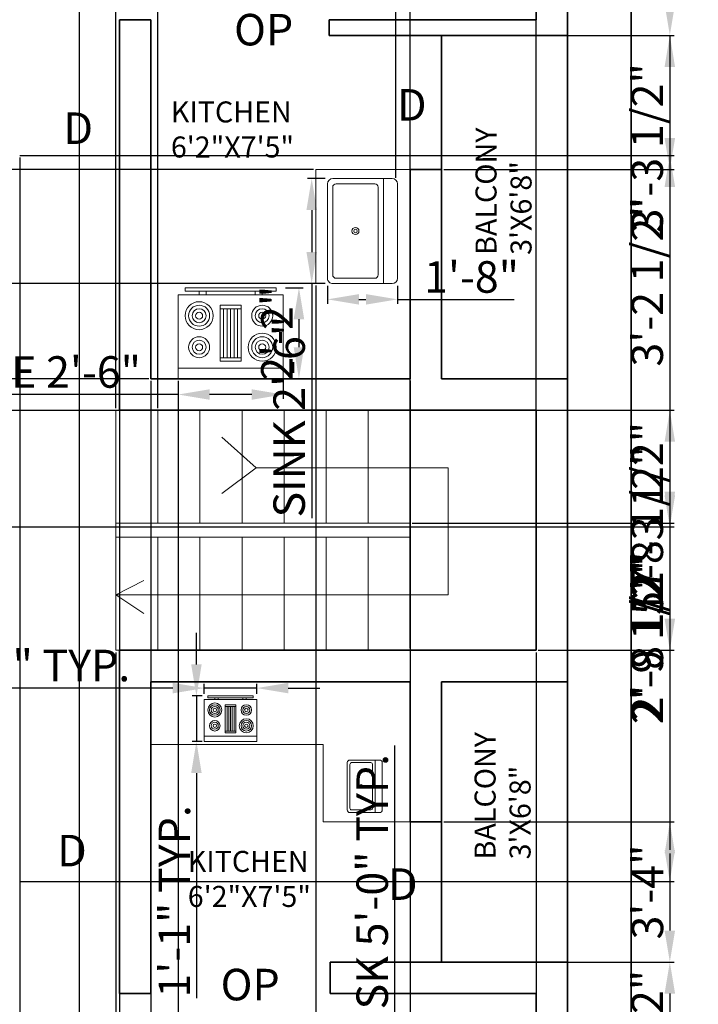
# Model space of a CAD drawing. Units: inches. Extents: x 53076 to 53578, y 41072 to 41816.
# Tile 3 of 4: x 53326 to 53520, y 41279 to 41560. Entities that reach past the tile are written whole.
import ezdxf

# ---------------------------------------------------------------- set-up
doc = ezdxf.new("R2010")
doc.units = ezdxf.units.IN
for name, color, linetype, lineweight in [('A-ANNO-DIMS', 2, 'Continuous', 18), ('A-ANNO-TEXT', 7, 'Continuous', 18), ('A-ANNO-TTLB', 7, 'Continuous', 35), ('A-AREA-IDEN', 7, 'Continuous', 18), ('A-DOOR', 3, 'Continuous', 25), ('A-EQPM', 8, 'Continuous', 18), ('A-FLOR-CASE', 9, 'Continuous', 18), ('A-FLOR-FIXT', 9, 'Continuous', 18), ('A-FLOR-STRS', 7, 'Continuous', 18), ('A-WALL', 7, 'Continuous', 35)]:
    doc.layers.add(name, color=color, linetype=linetype, lineweight=lineweight)
doc.styles.get("Standard").update_dxf_attribs({"font": 'arial.ttf'})
doc.dimstyles.new('ISO-25', dxfattribs={"dimtxt": 9, "dimasz": 9, "dimexe": 1.25, "dimexo": 0.625, "dimtad": 1, "dimdec": 1, "dimrnd": 9, "dimlunit": 3, "dimtxsty": 'Standard', "dimcen": 2.5, "dimadec": 0, "dimazin": 0, "dimtfac": 1, "dimtdec": 1, "dimtmove": 0, "dimatfit": 3, "dimfxl": 1, "dimarcsym": 0})

# ---------------------------------------------------------------- blocks, each defined once
blk = doc.blocks.new('Sink-single - 30 in top')
blk.add_line((-15, -3.999996), (15, -3.999996))
for points in [[(-13.5, 0), (13.5, 0)], [(-15, -18.499996), (-15, -1.5)], [(15, -1.5), (15, -18.499996)], [(-12.5, -5.499996), (12.5, -5.499996)], [(-13.5, -17.499996), (-13.5, -6.499996)], [(13.5, -6.499996), (13.5, -17.499996)], [(12.5, -18.499996), (-12.5, -18.499996)], [(13.5, -19.999996), (-13.5, -19.999996)]]:
    blk.add_lwpolyline(points)
for radius in [1, 0.5]:
    blk.add_circle((0, -11.999996), radius)
for centre, radius, start, end in [((-13.5, -1.5), 1.5, 90, 180), ((13.5, -1.5), 1.5, 0, 90), ((-12.5, -6.499996), 1, 90, 180), ((12.5, -6.499996), 1, 0, 90), ((-13.5, -18.499996), 1.5, 180, 270), ((-12.5, -17.499996), 1, 180, 270), ((12.5, -17.499996), 1, 270, 0), ((13.5, -18.499996), 1.5, 270, 0)]:
    blk.add_arc(centre, radius, start, end)
blk = doc.blocks.new('Range-Oven - 30 in top')
for p, q in [((0, -3), (30, -3)), ((12, -6), (18, -6)), ((13, -20), (13, -6)), ((14, -6), (14, -20)), ((15, -20), (15, -6)), ((16, -6), (16, -20)), ((17, -20), (17, -6)), ((18, -20), (12, -20)), ((6, -24), (6, -25)), ((8, -25), (8, -24)), ((22, -25), (22, -24)), ((24, -24), (24, -25))]:
    blk.add_line(p, q)
for points in [[(0, -24), (0, 0), (30, 0), (30, -24)], [(12, -21), (12, -5), (18, -5), (18, -21)], [(2, -26), (2, -25), (28, -25), (28, -26)]]:
    blk.add_lwpolyline(points, close=True)
for centre, radius in [((6, -9), 4), ((6, -9), 3), ((6, -9), 2), ((6, -9), 1), ((24, -9), 3), ((24, -9), 2), ((24, -9), 1), ((24, -18), 4), ((6, -18), 3), ((6, -18), 2), ((24, -18), 3), ((24, -18), 2), ((6, -18), 1), ((24, -18), 1)]:
    blk.add_circle(centre, radius)
blk = doc.blocks.new('DOOR-ENTRY-28_5IN')
blk.add_line((0, 0), (28.5, 0))
blk = doc.blocks.new('*D16')
at = {"layer": 'A-ANNO-DIMS', "color": 0, "lineweight": -2, "transparency": 16777216}
for p, q in [((53413.6, 41514.33), (53408.47, 41514.33)), ((53409.72, 41505.33), (53409.72, 41493.33)), ((53413.6, 41484.33), (53408.47, 41484.33)), ((53409.72, 41484.33), (53409.72, 41417.36))]:
    blk.add_line(p, q, dxfattribs=at)
at = {"layer": 'A-ANNO-DIMS', "color": 0, "transparency": 16777216}
for points in [[(53408.22, 41505.33), (53411.22, 41505.33), (53409.72, 41514.33)], [(53408.22, 41493.33), (53411.22, 41493.33), (53409.72, 41484.33)]]:
    blk.add_solid(points, dxfattribs=at)
at = {"layer": 'Defpoints', "color": 0, "transparency": 16777216}
for p in [(53414.22, 41514.33), (53409.72, 41484.33), (53414.22, 41484.33)]:
    blk.add_point(p, dxfattribs=at)
at = {"layer": 'A-ANNO-DIMS', "color": 0, "transparency": 16777216, "insert": (53404.44, 41446.35), "char_height": 9, "attachment_point": 5, "rotation": 90}
blk.add_mtext('SINK 2\'-6"', dxfattribs=at)
blk = doc.blocks.new('*D17')
at = {"layer": 'A-ANNO-DIMS', "color": 0, "lineweight": -2, "transparency": 16777216}
for p, q in [((53414.22, 41483.71), (53414.22, 41478.58)), ((53434.22, 41483.71), (53434.22, 41478.58)), ((53423.22, 41479.83), (53425.22, 41479.83)), ((53434.22, 41479.83), (53467.55, 41479.83))]:
    blk.add_line(p, q, dxfattribs=at)
at = {"layer": 'A-ANNO-DIMS', "color": 0, "transparency": 16777216}
for points in [[(53423.22, 41481.33), (53423.22, 41478.33), (53414.22, 41479.83)], [(53425.22, 41481.33), (53425.22, 41478.33), (53434.22, 41479.83)]]:
    blk.add_solid(points, dxfattribs=at)
at = {"layer": 'Defpoints', "color": 0, "transparency": 16777216}
for p in [(53414.22, 41484.33), (53434.22, 41484.33), (53434.22, 41479.83)]:
    blk.add_point(p, dxfattribs=at)
at = {"layer": 'A-ANNO-DIMS', "color": 0, "transparency": 16777216, "insert": (53455.38, 41485.05), "char_height": 9, "attachment_point": 5}
blk.add_mtext('1\'-8"', dxfattribs=at)
blk = doc.blocks.new('*D20')
at = {"layer": 'A-ANNO-DIMS', "color": 0, "lineweight": -2, "transparency": 16777216}
for p, q in [((53371.57, 41456.53), (53371.57, 41451.41)), ((53401.57, 41456.53), (53401.57, 41451.41)), ((53371.57, 41452.66), (53289.65, 41452.66)), ((53392.57, 41452.66), (53380.57, 41452.66))]:
    blk.add_line(p, q, dxfattribs=at)
at = {"layer": 'A-ANNO-DIMS', "color": 0, "transparency": 16777216}
for points in [[(53380.57, 41454.16), (53380.57, 41451.16), (53371.57, 41452.66)], [(53392.57, 41454.16), (53392.57, 41451.16), (53401.57, 41452.66)]]:
    blk.add_solid(points, dxfattribs=at)
at = {"layer": 'Defpoints', "color": 0, "transparency": 16777216}
for p in [(53371.57, 41457.16), (53401.57, 41457.16), (53371.57, 41452.66)]:
    blk.add_point(p, dxfattribs=at)
at = {"layer": 'A-ANNO-DIMS', "color": 0, "transparency": 16777216, "insert": (53326.11, 41457.93), "char_height": 9, "attachment_point": 5}
blk.add_mtext('RANGE 2\'-6"', dxfattribs=at)
blk = doc.blocks.new('*D21')
at = {"layer": 'A-ANNO-DIMS', "color": 0, "lineweight": -2, "transparency": 16777216}
for p, q in [((53402.19, 41483.16), (53407.32, 41483.16)), ((53406.07, 41474.16), (53406.07, 41466.16)), ((53402.19, 41457.16), (53407.32, 41457.16))]:
    blk.add_line(p, q, dxfattribs=at)
at = {"layer": 'A-ANNO-DIMS', "color": 0, "transparency": 16777216}
for points in [[(53404.57, 41474.16), (53407.57, 41474.16), (53406.07, 41483.16)], [(53404.57, 41466.16), (53407.57, 41466.16), (53406.07, 41457.16)]]:
    blk.add_solid(points, dxfattribs=at)
at = {"layer": 'Defpoints', "color": 0, "transparency": 16777216}
for p in [(53401.57, 41483.16), (53401.57, 41457.16), (53406.07, 41457.16)]:
    blk.add_point(p, dxfattribs=at)
at = {"layer": 'A-ANNO-DIMS', "color": 0, "transparency": 16777216, "insert": (53400.92, 41470.16), "char_height": 9, "attachment_point": 5, "rotation": 90}
blk.add_mtext('2\'-2"', dxfattribs=at)
blk = doc.blocks.new('*D22')
at = {"layer": 'A-ANNO-DIMS', "color": 0, "lineweight": -2, "transparency": 16777216}
for p, q in [((53379.04, 41367.23), (53379.04, 41370.11)), ((53394.04, 41367.23), (53394.04, 41370.11)), ((53370.04, 41368.86), (53257.19, 41368.86)), ((53394.04, 41368.86), (53379.04, 41368.86)), ((53403.04, 41368.86), (53412.04, 41368.86))]:
    blk.add_line(p, q, dxfattribs=at)
at = {"layer": 'A-ANNO-DIMS', "color": 0, "transparency": 16777216}
for points in [[(53370.04, 41370.36), (53370.04, 41367.36), (53379.04, 41368.86)], [(53403.04, 41370.36), (53403.04, 41367.36), (53394.04, 41368.86)]]:
    blk.add_solid(points, dxfattribs=at)
at = {"layer": 'Defpoints', "color": 0, "transparency": 16777216}
for p in [(53379.04, 41368.86), (53379.04, 41366.61), (53394.04, 41366.61)]:
    blk.add_point(p, dxfattribs=at)
at = {"layer": 'A-ANNO-DIMS', "color": 0, "transparency": 16777216, "insert": (53309.12, 41374.14), "char_height": 9, "attachment_point": 5}
blk.add_mtext('RANGE 1\'-3" TYP.', dxfattribs=at)
blk = doc.blocks.new('*D23')
at = {"layer": 'A-ANNO-DIMS', "color": 0, "lineweight": -2, "transparency": 16777216}
for p, q in [((53376.79, 41375.61), (53376.79, 41384.61)), ((53378.42, 41366.61), (53375.54, 41366.61)), ((53376.79, 41366.61), (53376.79, 41353.61)), ((53378.42, 41353.61), (53375.54, 41353.61)), ((53376.79, 41344.61), (53376.79, 41280.35))]:
    blk.add_line(p, q, dxfattribs=at)
at = {"layer": 'A-ANNO-DIMS', "color": 0, "transparency": 16777216}
for points in [[(53375.29, 41375.61), (53378.29, 41375.61), (53376.79, 41366.61)], [(53375.29, 41344.61), (53378.29, 41344.61), (53376.79, 41353.61)]]:
    blk.add_solid(points, dxfattribs=at)
at = {"layer": 'Defpoints', "color": 0, "transparency": 16777216}
for p in [(53379.04, 41366.61), (53376.79, 41353.61), (53379.04, 41353.61)]:
    blk.add_point(p, dxfattribs=at)
at = {"layer": 'A-ANNO-DIMS', "color": 0, "transparency": 16777216, "insert": (53371.65, 41307.98), "char_height": 9, "attachment_point": 5, "rotation": 90}
blk.add_mtext('1\'-1" TYP.', dxfattribs=at)
blk = doc.blocks.new('*D28')
at = {"layer": 'A-ANNO-DIMS', "color": 0, "lineweight": -2, "transparency": 16777216}
for p, q in [((53433.43, 41250.06), (53433.43, 41352.45)), ((53425.06, 41250.06), (53434.68, 41250.06)), ((53433.43, 41199.06), (53433.43, 41241.06)), ((53425.06, 41190.06), (53434.68, 41190.06))]:
    blk.add_line(p, q, dxfattribs=at)
at = {"layer": 'A-ANNO-DIMS', "color": 0, "transparency": 16777216}
for points in [[(53431.93, 41241.06), (53434.93, 41241.06), (53433.43, 41250.06)], [(53431.93, 41199.06), (53434.93, 41199.06), (53433.43, 41190.06)]]:
    blk.add_solid(points, dxfattribs=at)
at = {"layer": 'Defpoints', "color": 0, "transparency": 16777216}
for p in [(53424.43, 41250.06), (53433.43, 41250.06), (53424.43, 41190.06)]:
    blk.add_point(p, dxfattribs=at)
at = {"layer": 'A-ANNO-DIMS', "color": 0, "transparency": 16777216, "insert": (53428.16, 41305.75), "char_height": 9, "attachment_point": 5, "rotation": 90}
blk.add_mtext('DESK 5\'-0" TYP.', dxfattribs=at)
blk = doc.blocks.new('*D32')
at = {"layer": 'A-ANNO-DIMS', "color": 0, "lineweight": -2, "transparency": 16777216}
for p, q in [((53483.43, 41594.51), (53513.26, 41594.51)), ((53512.01, 41585.51), (53512.01, 41564.16)), ((53483.43, 41555.16), (53513.26, 41555.16)), ((53512.01, 41555.16), (53512.01, 41500.02))]:
    blk.add_line(p, q, dxfattribs=at)
at = {"layer": 'A-ANNO-DIMS', "color": 0, "transparency": 16777216}
for points in [[(53510.51, 41585.51), (53513.51, 41585.51), (53512.01, 41594.51)], [(53510.51, 41564.16), (53513.51, 41564.16), (53512.01, 41555.16)]]:
    blk.add_solid(points, dxfattribs=at)
at = {"layer": 'Defpoints', "color": 0, "transparency": 16777216}
for p in [(53482.81, 41594.51), (53482.81, 41555.16), (53512.01, 41555.16)]:
    blk.add_point(p, dxfattribs=at)
at = {"layer": 'A-ANNO-DIMS', "color": 0, "transparency": 16777216, "insert": (53506.72, 41523.09), "char_height": 9, "attachment_point": 5, "rotation": 90}
blk.add_mtext('3\'-3 1/2"', dxfattribs=at)
blk = doc.blocks.new('*D33')
at = {"layer": 'A-ANNO-DIMS', "color": 0, "lineweight": -2, "transparency": 16777216}
for p, q in [((53474.43, 41448.16), (53513.26, 41448.16)), ((53512.01, 41439.16), (53512.01, 41388.66)), ((53474.43, 41379.66), (53513.26, 41379.66))]:
    blk.add_line(p, q, dxfattribs=at)
at = {"layer": 'A-ANNO-DIMS', "color": 0, "transparency": 16777216}
for points in [[(53510.51, 41439.16), (53513.51, 41439.16), (53512.01, 41448.16)], [(53510.51, 41388.66), (53513.51, 41388.66), (53512.01, 41379.66)]]:
    blk.add_solid(points, dxfattribs=at)
at = {"layer": 'Defpoints', "color": 0, "transparency": 16777216}
for p in [(53473.81, 41448.16), (53473.81, 41379.66), (53512.01, 41379.66)]:
    blk.add_point(p, dxfattribs=at)
at = {"layer": 'A-ANNO-DIMS', "color": 0, "transparency": 16777216, "insert": (53506.73, 41413.91), "char_height": 9, "attachment_point": 5, "rotation": 90}
blk.add_mtext('5\'-8 1/2"', dxfattribs=at)
blk = doc.blocks.new('*D34')
at = {"layer": 'A-ANNO-DIMS', "color": 0, "lineweight": -2, "transparency": 16777216}
for p, q in [((53353.81, 41379.03), (53353.81, 41122.21)), ((53473.81, 41379.03), (53473.81, 41122.21)), ((53362.81, 41123.46), (53464.81, 41123.46))]:
    blk.add_line(p, q, dxfattribs=at)
at = {"layer": 'A-ANNO-DIMS', "color": 0, "transparency": 16777216}
for points in [[(53362.81, 41124.96), (53362.81, 41121.96), (53353.81, 41123.46)], [(53464.81, 41124.96), (53464.81, 41121.96), (53473.81, 41123.46)]]:
    blk.add_solid(points, dxfattribs=at)
at = {"layer": 'Defpoints', "color": 0, "transparency": 16777216}
for p in [(53353.81, 41379.66), (53473.81, 41379.66), (53473.81, 41123.46)]:
    blk.add_point(p, dxfattribs=at)
at = {"layer": 'A-ANNO-DIMS', "color": 0, "transparency": 16777216, "insert": (53413.81, 41128.68), "char_height": 9, "attachment_point": 5}
blk.add_mtext('10\'-0"', dxfattribs=at)
blk = doc.blocks.new('*D35')
at = {"layer": 'A-ANNO-DIMS', "color": 0, "lineweight": -2, "transparency": 16777216}
for p, q in [((53483.43, 41290.66), (53513.26, 41290.66)), ((53512.01, 41281.66), (53512.01, 41246.92)), ((53483.43, 41237.92), (53513.26, 41237.92))]:
    blk.add_line(p, q, dxfattribs=at)
at = {"layer": 'A-ANNO-DIMS', "color": 0, "transparency": 16777216}
for points in [[(53510.51, 41281.66), (53513.51, 41281.66), (53512.01, 41290.66)], [(53510.51, 41246.92), (53513.51, 41246.92), (53512.01, 41237.92)]]:
    blk.add_solid(points, dxfattribs=at)
at = {"layer": 'Defpoints', "color": 0, "transparency": 16777216}
for p in [(53482.81, 41290.66), (53482.81, 41237.92), (53512.01, 41237.92)]:
    blk.add_point(p, dxfattribs=at)
at = {"layer": 'A-ANNO-DIMS', "color": 0, "transparency": 16777216, "insert": (53506.73, 41264.29), "char_height": 9, "attachment_point": 5, "rotation": 90}
blk.add_mtext('4\'-4 1/2"', dxfattribs=at)
blk = doc.blocks.new('*D37')
at = {"layer": 'A-ANNO-DIMS', "color": 0, "lineweight": -2, "transparency": 16777216}
for p, q in [((53326.31, 41520.3), (53326.31, 41122.21)), ((53354.81, 41520.3), (53354.81, 41122.21)), ((53335.31, 41123.46), (53345.81, 41123.46)), ((53354.81, 41123.46), (53410.11, 41123.46))]:
    blk.add_line(p, q, dxfattribs=at)
at = {"layer": 'A-ANNO-DIMS', "color": 0, "transparency": 16777216}
for points in [[(53335.31, 41124.96), (53335.31, 41121.96), (53326.31, 41123.46)], [(53345.81, 41124.96), (53345.81, 41121.96), (53354.81, 41123.46)]]:
    blk.add_solid(points, dxfattribs=at)
at = {"layer": 'Defpoints', "color": 0, "transparency": 16777216}
for p in [(53326.31, 41520.92), (53354.81, 41520.92), (53354.81, 41123.46)]:
    blk.add_point(p, dxfattribs=at)
at = {"layer": 'A-ANNO-DIMS', "color": 0, "transparency": 16777216, "insert": (53386.96, 41128.73), "char_height": 9, "attachment_point": 5}
blk.add_mtext('2\'-4 1/2"', dxfattribs=at)
blk = doc.blocks.new('*D38')
at = {"layer": 'A-ANNO-DIMS', "color": 0, "lineweight": -2, "transparency": 16777216}
for p, q in [((53326.93, 41520.92), (53513.26, 41520.92)), ((53512.01, 41511.92), (53512.01, 41322.66)), ((53326.93, 41313.66), (53513.26, 41313.66))]:
    blk.add_line(p, q, dxfattribs=at)
at = {"layer": 'A-ANNO-DIMS', "color": 0, "transparency": 16777216}
for points in [[(53510.51, 41511.92), (53513.51, 41511.92), (53512.01, 41520.92)], [(53510.51, 41322.66), (53513.51, 41322.66), (53512.01, 41313.66)]]:
    blk.add_solid(points, dxfattribs=at)
at = {"layer": 'Defpoints', "color": 0, "transparency": 16777216}
for p in [(53326.31, 41520.92), (53326.31, 41313.66), (53512.01, 41313.66)]:
    blk.add_point(p, dxfattribs=at)
at = {"layer": 'A-ANNO-DIMS', "color": 0, "transparency": 16777216, "insert": (53506.72, 41417.29), "char_height": 9, "attachment_point": 5, "rotation": 90}
blk.add_mtext('17\'-3 1/2"', dxfattribs=at)
blk = doc.blocks.new('*D53')
at = {"layer": 'A-ANNO-DIMS', "color": 0, "lineweight": -2, "transparency": 16777216}
for p, q in [((53447.43, 41555.16), (53513.26, 41555.16)), ((53512.01, 41546.16), (53512.01, 41525.86)), ((53447.43, 41516.86), (53513.26, 41516.86)), ((53512.01, 41516.86), (53512.01, 41461.72))]:
    blk.add_line(p, q, dxfattribs=at)
at = {"layer": 'A-ANNO-DIMS', "color": 0, "transparency": 16777216}
for points in [[(53510.51, 41546.16), (53513.51, 41546.16), (53512.01, 41555.16)], [(53510.51, 41525.86), (53513.51, 41525.86), (53512.01, 41516.86)]]:
    blk.add_solid(points, dxfattribs=at)
at = {"layer": 'Defpoints', "color": 0, "transparency": 16777216}
for p in [(53446.81, 41555.16), (53446.81, 41516.86), (53512.01, 41516.86)]:
    blk.add_point(p, dxfattribs=at)
at = {"layer": 'A-ANNO-DIMS', "color": 0, "transparency": 16777216, "insert": (53506.72, 41484.79), "char_height": 9, "attachment_point": 5, "rotation": 90}
blk.add_mtext('3\'-2 1/2"', dxfattribs=at)
blk = doc.blocks.new('*D54')
at = {"layer": 'A-ANNO-DIMS', "color": 0, "lineweight": -2, "transparency": 16777216}
for p, q in [((53447.43, 41330.66), (53513.26, 41330.66)), ((53512.01, 41321.66), (53512.01, 41299.66)), ((53447.43, 41290.66), (53513.26, 41290.66))]:
    blk.add_line(p, q, dxfattribs=at)
at = {"layer": 'A-ANNO-DIMS', "color": 0, "transparency": 16777216}
for points in [[(53510.51, 41321.66), (53513.51, 41321.66), (53512.01, 41330.66)], [(53510.51, 41299.66), (53513.51, 41299.66), (53512.01, 41290.66)]]:
    blk.add_solid(points, dxfattribs=at)
at = {"layer": 'Defpoints', "color": 0, "transparency": 16777216}
for p in [(53446.81, 41330.66), (53446.81, 41290.66), (53512.01, 41290.66)]:
    blk.add_point(p, dxfattribs=at)
at = {"layer": 'A-ANNO-DIMS', "color": 0, "transparency": 16777216, "insert": (53506.78, 41310.66), "char_height": 9, "attachment_point": 5, "rotation": 90}
blk.add_mtext('3\'-4"', dxfattribs=at)
blk = doc.blocks.new('*D55')
at = {"layer": 'A-ANNO-DIMS', "color": 0, "lineweight": -2, "transparency": 16777216}
for p, q in [((53322.2, 41589.03), (53322.2, 41122.21)), ((53343.31, 41584.53), (53343.31, 41122.21)), ((53331.2, 41123.46), (53334.31, 41123.46)), ((53343.31, 41123.46), (53376.63, 41123.46))]:
    blk.add_line(p, q, dxfattribs=at)
at = {"layer": 'A-ANNO-DIMS', "color": 0, "transparency": 16777216}
for points in [[(53331.2, 41124.96), (53331.2, 41121.96), (53322.2, 41123.46)], [(53334.31, 41124.96), (53334.31, 41121.96), (53343.31, 41123.46)]]:
    blk.add_solid(points, dxfattribs=at)
at = {"layer": 'Defpoints', "color": 0, "transparency": 16777216}
for p in [(53322.2, 41589.66), (53343.31, 41585.16), (53343.31, 41123.46)]:
    blk.add_point(p, dxfattribs=at)
at = {"layer": 'A-ANNO-DIMS', "color": 0, "transparency": 16777216, "insert": (53364.47, 41128.68), "char_height": 9, "attachment_point": 5}
blk.add_mtext('1\'-9"', dxfattribs=at)
blk = doc.blocks.new('*D58')
at = {"layer": 'A-ANNO-DIMS', "color": 0, "lineweight": -2, "transparency": 16777216}
for p, q in [((53273.43, 41448.16), (53513.26, 41448.16)), ((53512.01, 41439.16), (53512.01, 41423.85)), ((53273.43, 41414.85), (53513.26, 41414.85)), ((53512.01, 41414.85), (53512.01, 41359.55))]:
    blk.add_line(p, q, dxfattribs=at)
at = {"layer": 'A-ANNO-DIMS', "color": 0, "transparency": 16777216}
for points in [[(53510.51, 41439.16), (53513.51, 41439.16), (53512.01, 41448.16)], [(53510.51, 41423.85), (53513.51, 41423.85), (53512.01, 41414.85)]]:
    blk.add_solid(points, dxfattribs=at)
at = {"layer": 'Defpoints', "color": 0, "transparency": 16777216}
for p in [(53272.81, 41448.16), (53272.81, 41414.85), (53512.01, 41414.85)]:
    blk.add_point(p, dxfattribs=at)
at = {"layer": 'A-ANNO-DIMS', "color": 0, "transparency": 16777216, "insert": (53506.73, 41382.7), "char_height": 9, "attachment_point": 5, "rotation": 90}
blk.add_mtext('2\'-9 1/2"', dxfattribs=at)
blk = doc.blocks.new('*D60')
at = {"layer": 'A-ANNO-DIMS', "color": 0, "lineweight": -2, "transparency": 16777216}
for p, q in [((53286.43, 41391.78), (53286.43, 41713.11)), ((53295.43, 41711.86), (53312.81, 41711.86)), ((53321.81, 41374.01), (53321.81, 41713.11)), ((53321.81, 41711.86), (53384.1, 41711.86))]:
    blk.add_line(p, q, dxfattribs=at)
at = {"layer": 'A-ANNO-DIMS', "color": 0, "transparency": 16777216}
for points in [[(53295.43, 41713.36), (53295.43, 41710.36), (53286.43, 41711.86)], [(53312.81, 41713.36), (53312.81, 41710.36), (53321.81, 41711.86)]]:
    blk.add_solid(points, dxfattribs=at)
at = {"layer": 'Defpoints', "color": 0, "transparency": 16777216}
for p in [(53321.81, 41711.86), (53286.43, 41391.16), (53321.81, 41373.39)]:
    blk.add_point(p, dxfattribs=at)
at = {"layer": 'A-ANNO-DIMS', "color": 0, "transparency": 16777216, "insert": (53357.45, 41717.13), "char_height": 9, "attachment_point": 5}
blk.add_mtext('2\'-11 1/2"', dxfattribs=at)
blk = doc.blocks.new('*D61')
at = {"layer": 'A-ANNO-DIMS', "color": 0, "lineweight": -2, "transparency": 16777216}
for p, q in [((53437.81, 41380.28), (53437.81, 41713.11)), ((53446.81, 41711.86), (53464.81, 41711.86)), ((53473.81, 41380.28), (53473.81, 41713.11))]:
    blk.add_line(p, q, dxfattribs=at)
at = {"layer": 'A-ANNO-DIMS', "color": 0, "transparency": 16777216}
for points in [[(53446.81, 41713.36), (53446.81, 41710.36), (53437.81, 41711.86)], [(53464.81, 41713.36), (53464.81, 41710.36), (53473.81, 41711.86)]]:
    blk.add_solid(points, dxfattribs=at)
at = {"layer": 'Defpoints', "color": 0, "transparency": 16777216}
for p in [(53473.81, 41711.86), (53437.81, 41379.66), (53473.81, 41379.66)]:
    blk.add_point(p, dxfattribs=at)
at = {"layer": 'A-ANNO-DIMS', "color": 0, "transparency": 16777216, "insert": (53455.81, 41717.08), "char_height": 9, "attachment_point": 5}
blk.add_mtext('3\'-0"', dxfattribs=at)
blk = doc.blocks.new('*D62')
at = {"layer": 'A-ANNO-DIMS', "color": 0, "lineweight": -2, "transparency": 16777216}
for p, q in [((53344.81, 41711.86), (53335.81, 41711.86)), ((53353.81, 41448.78), (53353.81, 41713.11)), ((53353.81, 41711.86), (53365.81, 41711.86)), ((53365.81, 41448.78), (53365.81, 41713.11)), ((53374.81, 41711.86), (53408.13, 41711.86))]:
    blk.add_line(p, q, dxfattribs=at)
at = {"layer": 'A-ANNO-DIMS', "color": 0, "transparency": 16777216}
for points in [[(53344.81, 41713.36), (53344.81, 41710.36), (53353.81, 41711.86)], [(53374.81, 41713.36), (53374.81, 41710.36), (53365.81, 41711.86)]]:
    blk.add_solid(points, dxfattribs=at)
at = {"layer": 'Defpoints', "color": 0, "transparency": 16777216}
for p in [(53365.81, 41711.86), (53353.81, 41448.16), (53365.81, 41448.16)]:
    blk.add_point(p, dxfattribs=at)
at = {"layer": 'A-ANNO-DIMS', "color": 0, "transparency": 16777216, "insert": (53395.97, 41717.08), "char_height": 9, "attachment_point": 5}
blk.add_mtext('1\'-0"', dxfattribs=at)
blk = doc.blocks.new('*D63')
at = {"layer": 'A-ANNO-DIMS', "color": 0, "lineweight": -2, "transparency": 16777216}
for p, q in [((53438.43, 41448.16), (53513.26, 41448.16)), ((53512.01, 41439.16), (53512.01, 41424.91)), ((53438.43, 41415.91), (53513.26, 41415.91)), ((53512.01, 41415.91), (53512.01, 41360.61))]:
    blk.add_line(p, q, dxfattribs=at)
at = {"layer": 'A-ANNO-DIMS', "color": 0, "transparency": 16777216}
for points in [[(53510.51, 41439.16), (53513.51, 41439.16), (53512.01, 41448.16)], [(53510.51, 41424.91), (53513.51, 41424.91), (53512.01, 41415.91)]]:
    blk.add_solid(points, dxfattribs=at)
at = {"layer": 'Defpoints', "color": 0, "transparency": 16777216}
for p in [(53437.81, 41448.16), (53437.81, 41415.91), (53512.01, 41415.91)]:
    blk.add_point(p, dxfattribs=at)
at = {"layer": 'A-ANNO-DIMS', "color": 0, "transparency": 16777216, "insert": (53506.73, 41383.76), "char_height": 9, "attachment_point": 5, "rotation": 90}
blk.add_mtext('2\'-8 1/2"', dxfattribs=at)
blk = doc.blocks.new('*D64')
at = {"layer": 'A-ANNO-DIMS', "color": 0, "lineweight": -2, "transparency": 16777216}
for p, q in [((53363.81, 41456.53), (53363.81, 41122.21)), ((53371.57, 41456.53), (53371.57, 41122.21)), ((53354.81, 41123.46), (53345.81, 41123.46)), ((53363.81, 41123.46), (53371.57, 41123.46)), ((53380.57, 41123.46), (53414.74, 41123.46))]:
    blk.add_line(p, q, dxfattribs=at)
at = {"layer": 'A-ANNO-DIMS', "color": 0, "transparency": 16777216}
for points in [[(53354.81, 41124.96), (53354.81, 41121.96), (53363.81, 41123.46)], [(53380.57, 41124.96), (53380.57, 41121.96), (53371.57, 41123.46)]]:
    blk.add_solid(points, dxfattribs=at)
at = {"layer": 'Defpoints', "color": 0, "transparency": 16777216}
for p in [(53363.81, 41457.16), (53371.57, 41457.16), (53371.57, 41123.46)]:
    blk.add_point(p, dxfattribs=at)
at = {"layer": 'A-ANNO-DIMS', "color": 0, "transparency": 16777216, "insert": (53402.15, 41128.68), "char_height": 9, "attachment_point": 5}
blk.add_mtext('0\'-8"', dxfattribs=at)
blk = doc.blocks.new('*D65')
at = {"layer": 'A-ANNO-DIMS', "color": 0, "lineweight": -2, "transparency": 16777216}
for p, q in [((53410.86, 41483.76), (53410.86, 41122.21)), ((53437.81, 41456.53), (53437.81, 41122.21)), ((53419.86, 41123.46), (53428.81, 41123.46))]:
    blk.add_line(p, q, dxfattribs=at)
at = {"layer": 'A-ANNO-DIMS', "color": 0, "transparency": 16777216}
for points in [[(53419.86, 41124.96), (53419.86, 41121.96), (53410.86, 41123.46)], [(53428.81, 41124.96), (53428.81, 41121.96), (53437.81, 41123.46)]]:
    blk.add_solid(points, dxfattribs=at)
at = {"layer": 'Defpoints', "color": 0, "transparency": 16777216}
for p in [(53410.86, 41484.39), (53437.81, 41457.16), (53437.81, 41123.46)]:
    blk.add_point(p, dxfattribs=at)
at = {"layer": 'A-ANNO-DIMS', "color": 0, "transparency": 16777216, "insert": (53424.33, 41128.68), "char_height": 9, "attachment_point": 5}
blk.add_mtext('2\'-3"', dxfattribs=at)
blk = doc.blocks.new('*D66')
at = {"layer": 'A-ANNO-DIMS', "color": 0, "lineweight": -2, "transparency": 16777216}
for p, q in [((53363.18, 41484.39), (53116.36, 41484.39)), ((53117.61, 41466.16), (53117.61, 41475.39)), ((53363.18, 41457.16), (53116.36, 41457.16))]:
    blk.add_line(p, q, dxfattribs=at)
at = {"layer": 'A-ANNO-DIMS', "color": 0, "transparency": 16777216}
for points in [[(53116.11, 41475.39), (53119.11, 41475.39), (53117.61, 41484.39)], [(53116.11, 41466.16), (53119.11, 41466.16), (53117.61, 41457.16)]]:
    blk.add_solid(points, dxfattribs=at)
at = {"layer": 'Defpoints', "color": 0, "transparency": 16777216}
for p in [(53117.61, 41484.39), (53363.81, 41484.39), (53363.81, 41457.16)]:
    blk.add_point(p, dxfattribs=at)
at = {"layer": 'A-ANNO-DIMS', "color": 0, "transparency": 16777216, "insert": (53112.38, 41470.77), "char_height": 9, "attachment_point": 5, "rotation": 90}
blk.add_mtext('2\'-3"', dxfattribs=at)
blk = doc.blocks.new('*D67')
at = {"layer": 'A-ANNO-DIMS', "color": 0, "lineweight": -2, "transparency": 16777216}
for p, q in [((53424.78, 41711.86), (53415.78, 41711.86)), ((53433.78, 41514.52), (53433.78, 41713.11)), ((53433.78, 41711.86), (53437.81, 41711.86)), ((53437.81, 41517.49), (53437.81, 41713.11)), ((53446.81, 41711.86), (53480.98, 41711.86))]:
    blk.add_line(p, q, dxfattribs=at)
at = {"layer": 'A-ANNO-DIMS', "color": 0, "transparency": 16777216}
for points in [[(53424.78, 41713.36), (53424.78, 41710.36), (53433.78, 41711.86)], [(53446.81, 41713.36), (53446.81, 41710.36), (53437.81, 41711.86)]]:
    blk.add_solid(points, dxfattribs=at)
at = {"layer": 'Defpoints', "color": 0, "transparency": 16777216}
for p in [(53437.81, 41711.86), (53437.81, 41516.86), (53433.78, 41513.89)]:
    blk.add_point(p, dxfattribs=at)
at = {"layer": 'A-ANNO-DIMS', "color": 0, "transparency": 16777216, "insert": (53468.39, 41717.08), "char_height": 9, "attachment_point": 5}
blk.add_mtext('0\'-4"', dxfattribs=at)
blk = doc.blocks.new('*D70')
at = {"layer": 'A-ANNO-DIMS', "color": 0, "lineweight": -2, "transparency": 16777216}
for p, q in [((53410.23, 41516.86), (53116.36, 41516.86)), ((53117.61, 41507.86), (53117.61, 41493.39)), ((53410.23, 41484.39), (53116.36, 41484.39)), ((53117.61, 41484.39), (53117.61, 41429.09))]:
    blk.add_line(p, q, dxfattribs=at)
at = {"layer": 'A-ANNO-DIMS', "color": 0, "transparency": 16777216}
for points in [[(53116.11, 41507.86), (53119.11, 41507.86), (53117.61, 41516.86)], [(53116.11, 41493.39), (53119.11, 41493.39), (53117.61, 41484.39)]]:
    blk.add_solid(points, dxfattribs=at)
at = {"layer": 'Defpoints', "color": 0, "transparency": 16777216}
for p in [(53410.86, 41516.86), (53117.61, 41484.39), (53410.86, 41484.39)]:
    blk.add_point(p, dxfattribs=at)
at = {"layer": 'A-ANNO-DIMS', "color": 0, "transparency": 16777216, "insert": (53112.33, 41452.24), "char_height": 9, "attachment_point": 5, "rotation": 90}
blk.add_mtext('2\'-8 1/2"', dxfattribs=at)

msp = doc.modelspace()

# ---------------------------------------------------------------- linework, layer by layer
at = {"layer": 'A-ANNO-TTLB'}
msp.add_lwpolyline([(53105.85, 41713.9), (53500.98, 41713.9), (53500.98, 41125.46), (53105.85, 41125.46)], close=True, dxfattribs=at)
at = {"layer": 'A-FLOR-CASE'}
for p, q in [((53437.81, 41516.86), (53410.86, 41516.86)), ((53410.86, 41516.86), (53410.86, 41484.39)), ((53410.86, 41484.39), (53363.81, 41484.39)), ((53412.97, 41352.8), (53363.81, 41352.8)), ((53412.97, 41330.66), (53412.97, 41352.8)), ((53437.81, 41330.66), (53412.97, 41330.66))]:
    msp.add_line(p, q, dxfattribs=at)
at = {"layer": 'A-FLOR-STRS'}
for p, q in [((53353.81, 41448.16), (53353.81, 41379.66)), ((53353.81, 41448.16), (53354.81, 41448.16)), ((53365.81, 41448.16), (53365.81, 41415.91)), ((53377.81, 41448.16), (53377.81, 41415.91)), ((53389.81, 41448.16), (53389.81, 41415.91)), ((53401.81, 41448.16), (53401.81, 41415.91)), ((53413.81, 41448.16), (53413.81, 41415.91)), ((53425.81, 41448.16), (53425.81, 41415.91)), ((53437.81, 41448.16), (53437.81, 41379.66)), ((53393.81, 41431.72), (53384.09, 41440.45)), ((53393.81, 41431.72), (53384.09, 41424.39)), ((53448.66, 41431.72), (53393.81, 41431.72)), ((53448.66, 41395.48), (53448.66, 41431.72)), ((53437.81, 41415.91), (53353.81, 41415.91)), ((53437.81, 41411.91), (53353.81, 41411.91)), ((53365.81, 41411.91), (53365.81, 41379.66)), ((53377.81, 41411.91), (53377.81, 41379.66)), ((53389.81, 41411.91), (53389.81, 41379.66)), ((53401.81, 41411.91), (53401.81, 41379.66)), ((53413.81, 41411.91), (53413.81, 41379.66)), ((53425.81, 41411.91), (53425.81, 41379.66)), ((53353.81, 41395.48), (53361.81, 41399.6)), ((53353.81, 41395.48), (53448.66, 41395.48)), ((53353.81, 41395.48), (53361.81, 41390.16)), ((53354.81, 41379.66), (53353.81, 41379.66))]:
    msp.add_line(p, q, dxfattribs=at)
at = {"layer": 'A-WALL'}
for p, q in [((53482.81, 41682.66), (53482.81, 41370.66)), ((53473.81, 41673.66), (53473.81, 41559.66)), ((53363.81, 41559.66), (53354.81, 41559.66)), ((53354.81, 41559.66), (53354.81, 41555.16)), ((53363.81, 41555.16), (53363.81, 41559.66)), ((53414.67, 41559.66), (53414.67, 41555.16)), ((53414.67, 41559.66), (53473.81, 41559.66)), ((53354.81, 41555.16), (53354.81, 41448.16)), ((53363.81, 41555.16), (53363.81, 41457.16)), ((53414.67, 41555.16), (53482.81, 41555.16)), ((53446.81, 41555.16), (53446.81, 41457.16)), ((53437.81, 41516.86), (53437.81, 41457.16)), ((53446.81, 41516.86), (53437.81, 41516.86)), ((53363.81, 41457.16), (53437.81, 41457.16)), ((53446.81, 41457.16), (53482.81, 41457.16)), ((53354.81, 41448.16), (53473.81, 41448.16)), ((53473.81, 41448.16), (53473.81, 41379.66)), ((53354.81, 41370.66), (53354.81, 41379.66)), ((53354.81, 41379.66), (53355.49, 41379.66)), ((53473.81, 41379.66), (53355.49, 41379.66)), ((53354.81, 41370.66), (53354.81, 41290.66)), ((53363.81, 41370.66), (53363.81, 41290.66)), ((53437.81, 41370.66), (53363.81, 41370.66)), ((53437.81, 41370.66), (53437.81, 41330.66)), ((53482.81, 41370.66), (53446.81, 41370.66)), ((53446.81, 41370.66), (53446.81, 41290.66)), ((53482.81, 41370.66), (53482.81, 41290.66)), ((53437.81, 41330.66), (53446.81, 41330.66)), ((53354.81, 41290.66), (53354.81, 41281.66)), ((53363.81, 41290.66), (53363.81, 41281.66)), ((53473.81, 41290.66), (53414.97, 41290.66)), ((53414.97, 41290.66), (53414.97, 41281.66)), ((53473.81, 41290.66), (53482.81, 41290.66)), ((53482.81, 41290.66), (53482.81, 41152.66)), ((53363.81, 41281.66), (53354.81, 41281.66)), ((53473.81, 41281.66), (53414.97, 41281.66)), ((53473.81, 41281.66), (53473.81, 41161.66))]:
    msp.add_line(p, q, dxfattribs=at)

# ---------------------------------------------------------------- block references
at = {"layer": 'A-DOOR'}
for p in [(53326.31, 41520.92), (53326.31, 41313.66)]:
    msp.add_blockref('DOOR-ENTRY-28_5IN', p, dxfattribs=at)
at = {"layer": 'A-EQPM', "rotation": 180}
msp.add_blockref('Range-Oven - 30 in top', (53401.57, 41457.16), dxfattribs=at)
at = {"layer": 'A-EQPM', "xscale": 0.5, "yscale": 0.5, "rotation": 180}
msp.add_blockref('Range-Oven - 30 in top', (53394.04, 41353.61), dxfattribs=at)
at = {"layer": 'A-FLOR-FIXT', "rotation": 270}
msp.add_blockref('Sink-single - 30 in top', (53434.22, 41499.33), dxfattribs=at)
at = {"layer": 'A-FLOR-FIXT', "xscale": 0.5, "yscale": 0.5, "rotation": 270}
msp.add_blockref('Sink-single - 30 in top', (53429.87, 41340.83), dxfattribs=at)

# ---------------------------------------------------------------- texts
at = {"layer": 'A-ANNO-TEXT', "char_height": 9, "attachment_point": 1}
for s, insert in [('OP ', (53387.55, 41561.31)), ('D ', (53434.08, 41539.85)), ('D ', (53338.82, 41533.18)), ('D ', (53337.02, 41326.97)), ('D ', (53431.53, 41317.41)), ('OP ', (53383.7, 41288.73))]:
    msp.add_mtext_dynamic_manual_height_columns(s, width=6.4326, gutter_width=12.5, heights=[0], dxfattribs=dict(at, insert=insert))
at = {"layer": 'A-AREA-IDEN', "char_height": 6, "attachment_point": 1}
for insert in [(53369.5, 41536.32), (53374.32, 41322.39)]:
    msp.add_mtext_dynamic_manual_height_columns('KITCHEN\\P6\'2"X7\'5"', width=85.6025, gutter_width=12.5, heights=[0], dxfattribs=dict(at, insert=insert))
at = {"layer": 'A-AREA-IDEN', "char_height": 6, "attachment_point": 1, "rotation": 90}
for insert in [(53456.51, 41492.52), (53456.24, 41319.96)]:
    msp.add_mtext_dynamic_manual_height_columns('BALCONY\\P3\'X6\'8"', width=85.6025, gutter_width=12.5, heights=[0], dxfattribs=dict(at, insert=insert))

# ---------------------------------------------------------------- dimensions: what is measured, and where the dimension line sits
at = {"layer": 'A-ANNO-DIMS'}
for base, p1, p2, picture, middle in [((53321.81, 41711.86), (53286.43, 41391.16), (53321.81, 41373.39), '*D60', (53357.45, 41717.13)), ((53365.81, 41711.86), (53353.81, 41448.16), (53365.81, 41448.16), '*D62', (53395.97, 41717.08)), ((53437.81, 41711.86), (53433.78, 41513.89), (53437.81, 41516.86), '*D67', (53468.39, 41717.08)), ((53473.81, 41711.86), (53437.81, 41379.66), (53473.81, 41379.66), '*D61', (53455.81, 41717.08)), ((53343.31, 41123.46), (53322.2, 41589.66), (53343.31, 41585.16), '*D55', (53364.47, 41128.68)), ((53354.81, 41123.46), (53326.31, 41520.92), (53354.81, 41520.92), '*D37', (53386.96, 41128.73)), ((53434.22, 41479.83), (53414.22, 41484.33), (53434.22, 41484.33), '*D17', (53455.38, 41485.05)), ((53437.8064, 41123.456), (53410.8553, 41484.3893), (53437.8064, 41457.156), '*D65', (53424.3308, 41128.6792)), ((53371.57, 41123.46), (53363.81, 41457.16), (53371.57, 41457.16), '*D64', (53402.15, 41128.68)), ((53473.81, 41123.46), (53353.81, 41379.66), (53473.81, 41379.66), '*D34', (53413.81, 41128.68))]:
    dim = msp.add_linear_dim(base=base, p1=p1, p2=p2, dimstyle='ISO-25', override={"dimdec": 1, "dimlfac": 1, "dimrnd": 0, "dimzin": 1, "dimdsep": 46, "dimlunit": 4, "dimfrac": 2}, dxfattribs=at)
    dim.commit()
    dim.dimension.update_dxf_attribs({"geometry": picture, "text_midpoint": middle})
for base, p1, p2, angle, picture, middle in [((53512.0064, 41555.156), (53482.8064, 41594.5051), (53482.8064, 41555.156), 90, '*D32', (53506.7248, 41523.0863)), ((53512.01, 41516.86), (53446.81, 41555.16), (53446.81, 41516.86), 90, '*D53', (53506.72, 41484.79)), ((53512.01, 41313.66), (53326.31, 41520.92), (53326.31, 41313.66), 90, '*D38', (53506.72, 41417.29)), ((53117.61, 41484.39), (53410.86, 41516.86), (53410.86, 41484.39), 90, '*D70', (53112.33, 41452.24)), ((53117.61, 41484.39), (53363.81, 41457.16), (53363.81, 41484.39), 90, '*D66', (53112.38, 41470.77)), ((53406.07, 41457.16), (53401.57, 41483.16), (53401.57, 41457.16), 270, '*D21', (53400.92, 41470.16)), ((53512.01, 41414.85), (53272.81, 41448.16), (53272.81, 41414.85), 90, '*D58', (53506.73, 41382.7)), ((53512.006388, 41415.906005), (53437.806388, 41448.156005), (53437.806388, 41415.906005), 90, '*D63', (53506.72790915, 41383.75644838)), ((53512.01, 41379.66), (53473.81, 41448.16), (53473.81, 41379.66), 90, '*D33', (53506.73, 41413.91)), ((53512.01, 41290.66), (53446.81, 41330.66), (53446.81, 41290.66), 90, '*D54', (53506.78, 41310.66)), ((53512.01, 41237.92), (53482.81, 41290.66), (53482.81, 41237.92), 90, '*D35', (53506.73, 41264.29))]:
    dim = msp.add_linear_dim(base=base, p1=p1, p2=p2, angle=angle, dimstyle='ISO-25', override={"dimdec": 1, "dimlfac": 1, "dimrnd": 0, "dimzin": 1, "dimdsep": 46, "dimlunit": 4, "dimfrac": 2}, dxfattribs=at)
    dim.commit()
    dim.dimension.update_dxf_attribs({"geometry": picture, "text_midpoint": middle})
for base, p1, p2, angle, text, picture, middle in [((53409.72, 41484.33), (53414.22, 41514.33), (53414.22, 41484.33), 270, 'SINK <>', '*D16', (53404.44, 41446.35)), ((53371.57, 41452.66), (53401.57, 41457.16), (53371.57, 41457.16), 180, 'RANGE <>', '*D20', (53326.11, 41457.93)), ((53379.04, 41368.86), (53394.04, 41366.61), (53379.04, 41366.61), 180, 'RANGE <> TYP.', '*D22', (53309.12, 41374.14)), ((53376.79, 41353.61), (53379.04, 41366.61), (53379.04, 41353.61), 270, '<> TYP.', '*D23', (53371.65, 41307.98)), ((53433.43, 41250.06), (53424.43, 41190.06), (53424.43, 41250.06), 90, 'DESK <> TYP.', '*D28', (53428.16, 41305.75))]:
    dim = msp.add_linear_dim(base=base, p1=p1, p2=p2, angle=angle, text=text, dimstyle='ISO-25', override={"dimdec": 1, "dimlfac": 1, "dimrnd": 0, "dimzin": 1, "dimdsep": 46, "dimlunit": 4, "dimfrac": 2}, dxfattribs=at)
    dim.commit()
    dim.dimension.update_dxf_attribs({"geometry": picture, "text_midpoint": middle})

doc.saveas('drawing.dxf')
